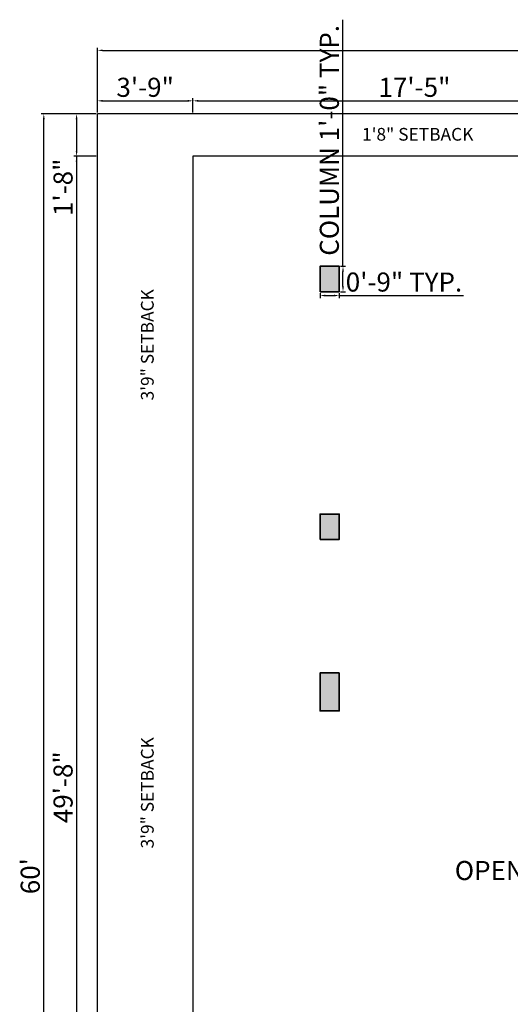
# Model space of a CAD drawing. Units: inches. Extents: x 3321 to 5237, y 11 to 1752.
# Tile 26 of 43: x 4649 to 4881, y 1287 to 1752. Entities that reach past the tile are written whole.
import ezdxf

# ---------------------------------------------------------------- set-up
doc = ezdxf.new("R2010")
doc.units = ezdxf.units.IN
for name, color, linetype, lineweight in [('A-ANNO-DIMS', 2, 'Continuous', 18), ('A-ANNO-TEXT', 7, 'Continuous', 18), ('A-AREA-IDEN', 7, 'Continuous', 18), ('A-COLS', 1, 'Continuous', 35), ('A-FLOR-EDGE', 7, 'Continuous', 25), ('C-PROP', 7, 'Continuous', 30)]:
    doc.layers.add(name, color=color, linetype=linetype, lineweight=lineweight)
doc.styles.get("Standard").update_dxf_attribs({"font": 'arial.ttf'})
doc.dimstyles.new('ISO-25', dxfattribs={"dimtxt": 9, "dimasz": 2.5, "dimexe": 1.25, "dimexo": 0.625, "dimtad": 1, "dimdec": 1, "dimlunit": 3, "dimtxsty": 'Standard', "dimcen": 2.5, "dimclrd": 4, "dimclre": 4, "dimclrt": 256, "dimadec": 0, "dimazin": 0, "dimtfac": 1, "dimtdec": 1, "dimtmove": 0, "dimatfit": 3, "dimfxl": 1, "dimarcsym": 0})

# ---------------------------------------------------------------- blocks, each defined once
blk = doc.blocks.new('*D12')
at = {"layer": 'A-ANNO-DIMS', "color": 0, "lineweight": -2, "transparency": 16777216}
for p, q in [((4686.08, 1707.96), (4686.08, 1714.75)), ((4688.58, 1713.5), (4728.58, 1713.5)), ((4731.08, 1707.96), (4731.08, 1714.75))]:
    blk.add_line(p, q, dxfattribs=at)
at = {"layer": 'A-ANNO-DIMS', "color": 0, "transparency": 16777216}
for points in [[(4688.58, 1713.92), (4688.58, 1713.08), (4686.08, 1713.5)], [(4728.58, 1713.92), (4728.58, 1713.08), (4731.08, 1713.5)]]:
    blk.add_solid(points, dxfattribs=at)
at = {"layer": 'Defpoints', "color": 0, "transparency": 16777216}
for p in [(4731.08, 1713.5), (4686.08, 1707.34), (4731.08, 1707.34)]:
    blk.add_point(p, dxfattribs=at)
at = {"layer": 'A-ANNO-DIMS', "color": 0, "transparency": 16777216, "insert": (4708.58, 1718.72), "char_height": 9, "attachment_point": 5}
blk.add_mtext('3\'-9"', dxfattribs=at)
blk = doc.blocks.new('*D13')
at = {"layer": 'A-ANNO-DIMS', "color": 0, "lineweight": -2, "transparency": 16777216}
for p, q in [((4731.08, 1707.96), (4731.08, 1714.75)), ((4733.58, 1713.5), (4937.58, 1713.5)), ((4940.08, 1707.96), (4940.08, 1714.75))]:
    blk.add_line(p, q, dxfattribs=at)
at = {"layer": 'A-ANNO-DIMS', "color": 0, "transparency": 16777216}
for points in [[(4733.58, 1713.92), (4733.58, 1713.08), (4731.08, 1713.5)], [(4937.58, 1713.92), (4937.58, 1713.08), (4940.08, 1713.5)]]:
    blk.add_solid(points, dxfattribs=at)
at = {"layer": 'Defpoints', "color": 0, "transparency": 16777216}
for p in [(4940.08, 1713.5), (4731.08, 1707.34), (4940.08, 1707.34)]:
    blk.add_point(p, dxfattribs=at)
at = {"layer": 'A-ANNO-DIMS', "color": 0, "transparency": 16777216, "insert": (4835.58, 1718.72), "char_height": 9, "attachment_point": 5}
blk.add_mtext('17\'-5"', dxfattribs=at)
blk = doc.blocks.new('*D16')
at = {"layer": 'A-ANNO-DIMS', "color": 0, "lineweight": -2, "transparency": 16777216}
for p, q in [((4685.46, 1707.34), (4674.99, 1707.34)), ((4676.24, 1704.84), (4676.24, 1689.84)), ((4685.46, 1687.34), (4674.99, 1687.34)), ((4676.24, 1687.34), (4676.24, 1660.51))]:
    blk.add_line(p, q, dxfattribs=at)
at = {"layer": 'A-ANNO-DIMS', "color": 0, "transparency": 16777216}
for points in [[(4675.82, 1704.84), (4676.66, 1704.84), (4676.24, 1707.34)], [(4675.82, 1689.84), (4676.66, 1689.84), (4676.24, 1687.34)]]:
    blk.add_solid(points, dxfattribs=at)
at = {"layer": 'Defpoints', "color": 0, "transparency": 16777216}
for p in [(4686.08, 1707.34), (4676.24, 1687.34), (4686.08, 1687.34)]:
    blk.add_point(p, dxfattribs=at)
at = {"layer": 'A-ANNO-DIMS', "color": 0, "transparency": 16777216, "insert": (4671.02, 1672.67), "char_height": 9, "attachment_point": 5, "rotation": 90}
blk.add_mtext('1\'-8"', dxfattribs=at)
blk = doc.blocks.new('*D17')
at = {"layer": 'A-ANNO-DIMS', "color": 0, "lineweight": -2, "transparency": 16777216}
for p, q in [((4685.46, 1687.34), (4674.99, 1687.34)), ((4676.24, 1684.84), (4676.24, 1093.84)), ((4685.46, 1091.34), (4674.99, 1091.34))]:
    blk.add_line(p, q, dxfattribs=at)
at = {"layer": 'A-ANNO-DIMS', "color": 0, "transparency": 16777216}
for points in [[(4675.82, 1684.84), (4676.66, 1684.84), (4676.24, 1687.34)], [(4675.82, 1093.84), (4676.66, 1093.84), (4676.24, 1091.34)]]:
    blk.add_solid(points, dxfattribs=at)
at = {"layer": 'Defpoints', "color": 0, "transparency": 16777216}
for p in [(4686.08, 1687.34), (4676.24, 1091.34), (4686.08, 1091.34)]:
    blk.add_point(p, dxfattribs=at)
at = {"layer": 'A-ANNO-DIMS', "color": 0, "transparency": 16777216, "insert": (4671.02, 1389.34), "char_height": 9, "attachment_point": 5, "rotation": 90}
blk.add_mtext('49\'-8"', dxfattribs=at)
blk = doc.blocks.new('*D29')
at = {"layer": 'A-ANNO-DIMS', "color": 0, "lineweight": -2, "transparency": 16777216}
for p, q in [((4685.46, 1707.34), (4659.51, 1707.34)), ((4660.76, 989.84), (4660.76, 1704.84)), ((4685.46, 987.34), (4659.51, 987.34))]:
    blk.add_line(p, q, dxfattribs=at)
at = {"layer": 'A-ANNO-DIMS', "color": 0, "transparency": 16777216}
for points in [[(4660.35, 1704.84), (4661.18, 1704.84), (4660.76, 1707.34)], [(4660.35, 989.84), (4661.18, 989.84), (4660.76, 987.34)]]:
    blk.add_solid(points, dxfattribs=at)
at = {"layer": 'Defpoints', "color": 0, "transparency": 16777216}
for p in [(4660.76, 1707.34), (4686.08, 1707.34), (4686.08, 987.34)]:
    blk.add_point(p, dxfattribs=at)
at = {"layer": 'A-ANNO-DIMS', "color": 0, "transparency": 16777216, "insert": (4655.54, 1347.34), "char_height": 9, "attachment_point": 5, "rotation": 90}
blk.add_mtext("60'", dxfattribs=at)
blk = doc.blocks.new('*D149')
at = {"layer": 'A-ANNO-DIMS', "color": 0, "lineweight": -2, "transparency": 16777216}
for p, q in [((4686.08, 1707.96), (4686.08, 1738.58)), ((4688.58, 1737.33), (5163.58, 1737.33)), ((5166.08, 1707.96), (5166.08, 1738.58))]:
    blk.add_line(p, q, dxfattribs=at)
at = {"layer": 'A-ANNO-DIMS', "color": 0, "transparency": 16777216}
for points in [[(4688.58, 1737.74), (4688.58, 1736.91), (4686.08, 1737.33)], [(5163.58, 1737.74), (5163.58, 1736.91), (5166.08, 1737.33)]]:
    blk.add_solid(points, dxfattribs=at)
at = {"layer": 'Defpoints', "color": 0, "transparency": 16777216}
for p in [(5166.08, 1737.33), (4686.08, 1707.34), (5166.08, 1707.34)]:
    blk.add_point(p, dxfattribs=at)
at = {"layer": 'A-ANNO-DIMS', "color": 0, "transparency": 16777216, "insert": (4926.08, 1742.55), "char_height": 9, "attachment_point": 5}
blk.add_mtext("40'", dxfattribs=at)
blk = doc.blocks.new('COL-9X18-IN')
h = blk.add_hatch(color=256)
h.dxf.hatch_style = 1
h.paths.add_polyline_path([(9, 18), (0, 18), (0, 0), (9, 0)])
blk.add_lwpolyline([(0, 0), (9, 0), (9, 18), (0, 18)], close=True)
blk = doc.blocks.new('COL-9X12-FURN-PLAN')
h = blk.add_hatch(color=256)
h.dxf.hatch_style = 1
h.paths.add_polyline_path([(0, 12), (0, 0), (9, 0), (9, 12)])
blk.add_lwpolyline([(0, 0), (9, 0), (9, 12), (0, 12)], close=True)
blk = doc.blocks.new('PROPERTY-40X60FT')
for p in [(480, 720), (0, 0)]:
    blk.add_line(p, (480, 0))
blk = doc.blocks.new('*D177')
at = {"layer": 'A-ANNO-DIMS', "color": 4, "lineweight": -2, "transparency": 16777216}
for p, q in [((4801.88, 1635.34), (4801.88, 1751.82)), ((4800.71, 1635.34), (4803.13, 1635.34)), ((4801.88, 1625.84), (4801.88, 1632.84)), ((4800.71, 1623.34), (4803.13, 1623.34))]:
    blk.add_line(p, q, dxfattribs=at)
at = {"layer": 'A-ANNO-DIMS', "color": 4, "transparency": 16777216}
for points in [[(4801.47, 1632.84), (4802.3, 1632.84), (4801.88, 1635.34)], [(4801.47, 1625.84), (4802.3, 1625.84), (4801.88, 1623.34)]]:
    blk.add_solid(points, dxfattribs=at)
at = {"layer": 'Defpoints', "color": 0, "transparency": 16777216}
for p in [(4800.08, 1635.34), (4801.88, 1635.34), (4800.08, 1623.34)]:
    blk.add_point(p, dxfattribs=at)
at = {"layer": 'A-ANNO-DIMS', "transparency": 16777216, "insert": (4796.6, 1694.83), "char_height": 9, "attachment_point": 5, "rotation": 90}
blk.add_mtext('COLUMN 1\'-0" TYP.', dxfattribs=at)
blk = doc.blocks.new('*D178')
at = {"layer": 'A-ANNO-DIMS', "color": 4, "lineweight": -2, "transparency": 16777216}
for p, q in [((4791.08, 1622.71), (4791.08, 1620.29)), ((4793.58, 1621.54), (4797.58, 1621.54)), ((4800.08, 1622.71), (4800.08, 1620.29)), ((4800.08, 1621.54), (4858.69, 1621.54))]:
    blk.add_line(p, q, dxfattribs=at)
at = {"layer": 'A-ANNO-DIMS', "color": 4, "transparency": 16777216}
for points in [[(4793.58, 1621.96), (4793.58, 1621.12), (4791.08, 1621.54)], [(4797.58, 1621.96), (4797.58, 1621.12), (4800.08, 1621.54)]]:
    blk.add_solid(points, dxfattribs=at)
at = {"layer": 'Defpoints', "color": 0, "transparency": 16777216}
for p in [(4791.08, 1623.34), (4800.08, 1623.34), (4800.08, 1621.54)]:
    blk.add_point(p, dxfattribs=at)
at = {"layer": 'A-ANNO-DIMS', "transparency": 16777216, "insert": (4830.64, 1626.76), "char_height": 9, "attachment_point": 5}
blk.add_mtext('0\'-9" TYP.', dxfattribs=at)

msp = doc.modelspace()

# ---------------------------------------------------------------- linework, layer by layer
at = {"layer": 'A-COLS'}
for p, q in [((4791.08, 1443.34), (4800.08, 1443.34)), ((4800.08, 1443.34), (4800.08, 1434.34))]:
    msp.add_line(p, q, dxfattribs=at)
at = {"layer": 'A-FLOR-EDGE'}
for p, q in [((4731.08, 1687.34), (4731.08, 1091.34)), ((5130.08, 1687.34), (4731.08, 1687.34))]:
    msp.add_line(p, q, dxfattribs=at)

# ---------------------------------------------------------------- block references
at = {"layer": 'A-COLS'}
for p in [(4791.08, 1623.34), (4791.08, 1506.34)]:
    msp.add_blockref('COL-9X12-FURN-PLAN', p, dxfattribs=at)
at = {"layer": 'A-COLS', "rotation": 180}
msp.add_blockref('COL-9X18-IN', (4800.08, 1443.34), dxfattribs=at)
at = {"layer": 'C-PROP', "rotation": 180}
msp.add_blockref('PROPERTY-40X60FT', (5166.08, 1707.34), dxfattribs=at)

# ---------------------------------------------------------------- texts
at = {"layer": 'A-ANNO-TEXT', "insert": (4810.85, 1700.7), "char_height": 6, "attachment_point": 1}
msp.add_mtext_dynamic_manual_height_columns('1\'8" SETBACK', width=97.3114, gutter_width=25, heights=[0], dxfattribs=at)
at = {"layer": 'A-ANNO-TEXT', "char_height": 6, "attachment_point": 1, "rotation": 90}
for insert in [(4706.6, 1572.02), (4706.6, 1360.44)]:
    msp.add_mtext_dynamic_manual_height_columns('3\'9" SETBACK', width=97.3114, gutter_width=25, heights=[0], dxfattribs=dict(at, insert=insert))
at = {"layer": 'A-AREA-IDEN', "insert": (4854.62, 1354.51), "char_height": 9, "attachment_point": 1}
msp.add_mtext_dynamic_manual_height_columns('OPEN TERRACE', width=123.9378, gutter_width=25, heights=[0], dxfattribs=at)

# ---------------------------------------------------------------- dimensions: what is measured, and where the dimension line sits
at = {"layer": 'A-ANNO-DIMS'}
for base, p1, p2, picture, middle in [((5166.08, 1737.33), (4686.08, 1707.34), (5166.08, 1707.34), '*D149', (4926.08, 1742.55)), ((4731.08, 1713.5), (4686.08, 1707.34), (4731.08, 1707.34), '*D12', (4708.58, 1718.72)), ((4940.08, 1713.5), (4731.08, 1707.34), (4940.08, 1707.34), '*D13', (4835.58, 1718.72))]:
    dim = msp.add_linear_dim(base=base, p1=p1, p2=p2, dimstyle='ISO-25', override={"dimclrd": 0, "dimclre": 0, "dimclrt": 0}, dxfattribs=at)
    dim.commit()
    dim.dimension.update_dxf_attribs({"geometry": picture, "text_midpoint": middle})
dim = msp.add_linear_dim(base=(4801.88, 1635.34), p1=(4800.08, 1623.34), p2=(4800.08, 1635.34), angle=90, text='COLUMN <> TYP.', dimstyle='ISO-25', override={"dimdec": 1, "dimlfac": 1, "dimrnd": 0, "dimzin": 1, "dimdsep": 46, "dimlunit": 4, "dimfrac": 2}, dxfattribs=at)
dim.commit()
dim.dimension.update_dxf_attribs({"geometry": '*D177', "text_midpoint": (4796.6, 1694.83)})
for base, p1, p2, picture, middle in [((4660.76, 1707.34), (4686.08, 987.34), (4686.08, 1707.34), '*D29', (4655.54, 1347.34)), ((4676.24, 1687.34), (4686.08, 1707.34), (4686.08, 1687.34), '*D16', (4671.02, 1672.67)), ((4676.24, 1091.34), (4686.08, 1687.34), (4686.08, 1091.34), '*D17', (4671.02, 1389.34))]:
    dim = msp.add_linear_dim(base=base, p1=p1, p2=p2, angle=90, dimstyle='ISO-25', override={"dimclrd": 0, "dimclre": 0, "dimclrt": 0}, dxfattribs=at)
    dim.commit()
    dim.dimension.update_dxf_attribs({"geometry": picture, "text_midpoint": middle})
dim = msp.add_linear_dim(base=(4800.08, 1621.54), p1=(4791.08, 1623.34), p2=(4800.08, 1623.34), text='<> TYP.', dimstyle='ISO-25', override={"dimdec": 1, "dimlfac": 1, "dimrnd": 0, "dimzin": 1, "dimdsep": 46, "dimlunit": 4, "dimfrac": 2}, dxfattribs=at)
dim.commit()
dim.dimension.update_dxf_attribs({"geometry": '*D178', "text_midpoint": (4830.64, 1626.76)})

doc.saveas('drawing.dxf')
